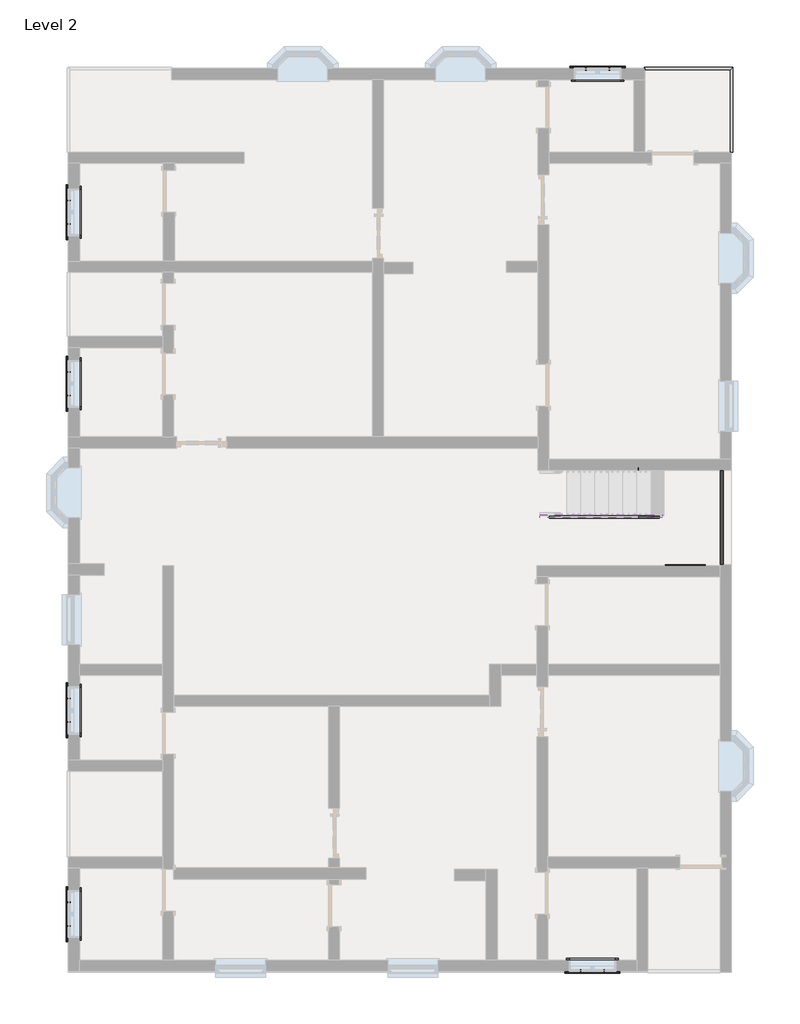
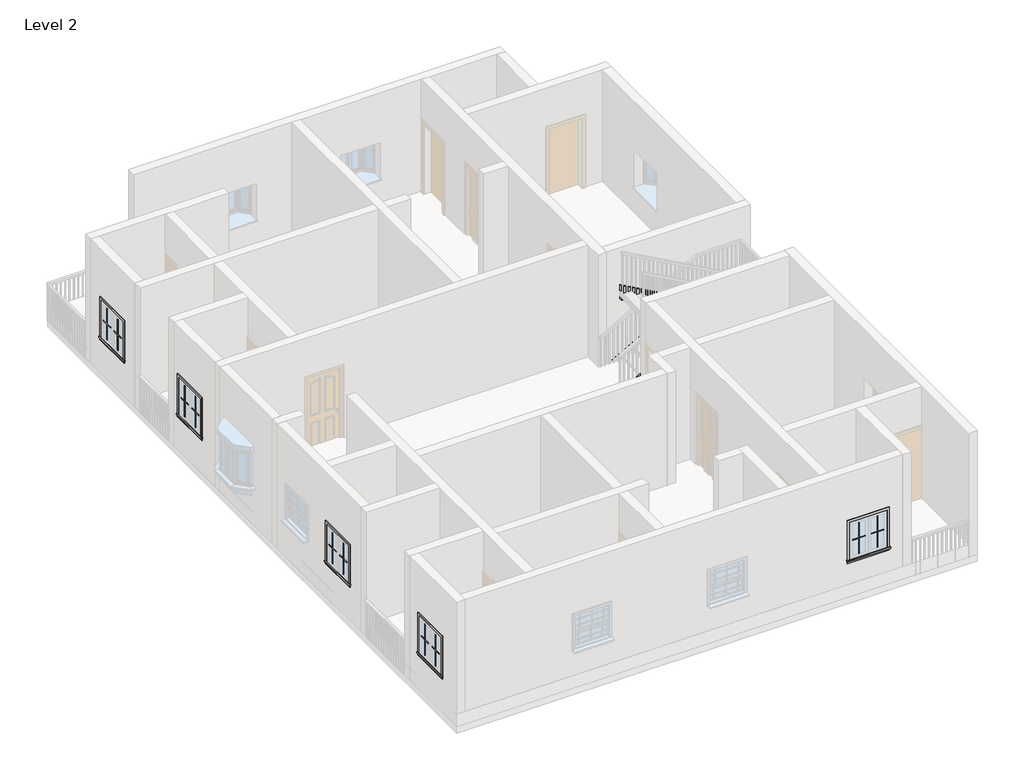
# One storey, part 4 of 4: 24 proxies, 5 members, 1 railing.
"""IFC4 building model written with IfcOpenShell, lengths in millimetres."""

from ifc_helpers import new_model, si_unit, frame, origin, place, context, project, spatial, polyline, outline, extrude, faceted_brep, transform, mapped, element, save
from components import muntin_pattern_2x2_muntin_pattern_2x2_b3fe6957, muntin_pattern_2x2_muntin_pattern_2x2_3e0ecaf2, trim_window_exterior_flat_with_sill_41619996, trim_window_interior_flat_picture_frame_51c85655

model = new_model("IFC4")

# Units and contexts
model_context = context("Model", 3, world=origin())
ifc_project = project(units=[si_unit("LENGTHUNIT", "METRE", prefix="MILLI")], contexts=[model_context])

# Site, building, storey
site = spatial("IfcSite", under=ifc_project)
building = spatial("IfcBuilding", under=site)
storey = spatial("IfcBuildingStorey", under=building, Name="Level 2", Elevation=3048.0)

# Proxies
placement = place(None, origin())
muntin_pattern_2x2_muntin_pattern_2x2_shape = muntin_pattern_2x2_muntin_pattern_2x2_b3fe6957(model_context)
element("IfcBuildingElementProxy", 1, Name="Muntin Pattern_2x2 : Muntin Pattern_2x2", ObjectType="Muntin Pattern_2x2 : Muntin Pattern_2x2", at=placement, inside=storey, context=model_context, shape_type="MappedRepresentation", body=[
    mapped(muntin_pattern_2x2_muntin_pattern_2x2_shape, transform((-7038.4808717, 5489.0318597, 4032.25), x_axis=(0.0, 1.0, 0.0), y_axis=(-1.0, 0.0, 0.0), z_axis=(0.0, 0.0, 1.0))),
])
element("IfcBuildingElementProxy", 2, Name="Muntin Pattern_2x2 : Muntin Pattern_2x2", ObjectType="Muntin Pattern_2x2 : Muntin Pattern_2x2", at=placement, inside=storey, context=model_context, shape_type="MappedRepresentation", body=[
    mapped(muntin_pattern_2x2_muntin_pattern_2x2_shape, transform((-7038.4808717, 2366.9422293, 4032.25), x_axis=(0.0, 1.0, 0.0), y_axis=(-1.0, 0.0, 0.0), z_axis=(0.0, 0.0, 1.0))),
])
element("IfcBuildingElementProxy", 3, Name="Muntin Pattern_2x2 : Muntin Pattern_2x2", ObjectType="Muntin Pattern_2x2 : Muntin Pattern_2x2", at=placement, inside=storey, context=model_context, shape_type="MappedRepresentation", body=[
    mapped(muntin_pattern_2x2_muntin_pattern_2x2_shape, transform((2376.9816283, 8312.1297293, 4032.25), x_axis=(1.0, 0.0, 0.0), y_axis=(0.0, 1.0, 0.0), z_axis=(0.0, 0.0, 1.0))),
])
element("IfcBuildingElementProxy", 4, Name="Muntin Pattern_2x2 : Muntin Pattern_2x2", ObjectType="Muntin Pattern_2x2 : Muntin Pattern_2x2", at=placement, inside=storey, context=model_context, shape_type="MappedRepresentation", body=[
    mapped(muntin_pattern_2x2_muntin_pattern_2x2_shape, transform((2710.3566283, -8102.6202707, 4032.25), x_axis=(-1.0, 0.0, 0.0), y_axis=(0.0, -1.0, 0.0), z_axis=(0.0, 0.0, 1.0))),
])
element("IfcBuildingElementProxy", 5, Name="Muntin Pattern_2x2 : Muntin Pattern_2x2", ObjectType="Muntin Pattern_2x2 : Muntin Pattern_2x2", at=placement, inside=storey, context=model_context, shape_type="MappedRepresentation", body=[
    mapped(muntin_pattern_2x2_muntin_pattern_2x2_shape, transform((-7038.4808717, -7285.0577707, 4032.25), x_axis=(0.0, 1.0, 0.0), y_axis=(-1.0, 0.0, 0.0), z_axis=(0.0, 0.0, 1.0))),
])
element("IfcBuildingElementProxy", 6, Name="Muntin Pattern_2x2 : Muntin Pattern_2x2", ObjectType="Muntin Pattern_2x2 : Muntin Pattern_2x2", at=placement, inside=storey, context=model_context, shape_type="MappedRepresentation", body=[
    mapped(muntin_pattern_2x2_muntin_pattern_2x2_shape, transform((-7038.4808717, -3576.6577707, 4032.25), x_axis=(0.0, 1.0, 0.0), y_axis=(-1.0, 0.0, 0.0), z_axis=(0.0, 0.0, 1.0))),
])
muntin_pattern_2x2_muntin_pattern_2x2_2_shape = muntin_pattern_2x2_muntin_pattern_2x2_3e0ecaf2(model_context)
element("IfcBuildingElementProxy", 7, Name="Muntin Pattern_2x2 : Muntin Pattern_2x2", ObjectType="Muntin Pattern_2x2 : Muntin Pattern_2x2", at=placement, inside=storey, context=model_context, shape_type="MappedRepresentation", body=[
    mapped(muntin_pattern_2x2_muntin_pattern_2x2_2_shape, transform((-7038.4808717, 5917.6568597, 4032.25), x_axis=(0.0, -1.0, 0.0), y_axis=(1.0, 0.0, 0.0), z_axis=(0.0, 0.0, 1.0))),
])
element("IfcBuildingElementProxy", 8, Name="Muntin Pattern_2x2 : Muntin Pattern_2x2", ObjectType="Muntin Pattern_2x2 : Muntin Pattern_2x2", at=placement, inside=storey, context=model_context, shape_type="MappedRepresentation", body=[
    mapped(muntin_pattern_2x2_muntin_pattern_2x2_2_shape, transform((-7038.4808717, 2795.5672293, 4032.25), x_axis=(0.0, -1.0, 0.0), y_axis=(1.0, 0.0, 0.0), z_axis=(0.0, 0.0, 1.0))),
])
element("IfcBuildingElementProxy", 9, Name="Muntin Pattern_2x2 : Muntin Pattern_2x2", ObjectType="Muntin Pattern_2x2 : Muntin Pattern_2x2", at=placement, inside=storey, context=model_context, shape_type="MappedRepresentation", body=[
    mapped(muntin_pattern_2x2_muntin_pattern_2x2_2_shape, transform((2805.6066283, 8312.1297293, 4032.25), x_axis=(-1.0, 0.0, 0.0), y_axis=(0.0, -1.0, 0.0), z_axis=(0.0, 0.0, 1.0))),
])
element("IfcBuildingElementProxy", 10, Name="Muntin Pattern_2x2 : Muntin Pattern_2x2", ObjectType="Muntin Pattern_2x2 : Muntin Pattern_2x2", at=placement, inside=storey, context=model_context, shape_type="MappedRepresentation", body=[
    mapped(muntin_pattern_2x2_muntin_pattern_2x2_2_shape, transform((2281.7316283, -8102.6202707, 4032.25), x_axis=(1.0, 0.0, 0.0), y_axis=(0.0, 1.0, 0.0), z_axis=(0.0, 0.0, 1.0))),
])
element("IfcBuildingElementProxy", 11, Name="Muntin Pattern_2x2 : Muntin Pattern_2x2", ObjectType="Muntin Pattern_2x2 : Muntin Pattern_2x2", at=placement, inside=storey, context=model_context, shape_type="MappedRepresentation", body=[
    mapped(muntin_pattern_2x2_muntin_pattern_2x2_2_shape, transform((-7038.4808717, -6856.4327707, 4032.25), x_axis=(0.0, -1.0, 0.0), y_axis=(1.0, 0.0, 0.0), z_axis=(0.0, 0.0, 1.0))),
])
element("IfcBuildingElementProxy", 12, Name="Muntin Pattern_2x2 : Muntin Pattern_2x2", ObjectType="Muntin Pattern_2x2 : Muntin Pattern_2x2", at=placement, inside=storey, context=model_context, shape_type="MappedRepresentation", body=[
    mapped(muntin_pattern_2x2_muntin_pattern_2x2_2_shape, transform((-7038.4808717, -3148.0327707, 4032.25), x_axis=(0.0, -1.0, 0.0), y_axis=(1.0, 0.0, 0.0), z_axis=(0.0, 0.0, 1.0))),
])
trim_window_exterior_flat_with_sill_shape = trim_window_exterior_flat_with_sill_41619996(model_context)
element("IfcBuildingElementProxy", 13, Name="Trim-Window-Exterior-Flat : with Sill", ObjectType="Trim-Window-Exterior-Flat : with Sill", at=placement, inside=storey, context=model_context, shape_type="MappedRepresentation", body=[
    mapped(trim_window_exterior_flat_with_sill_shape, transform((-7048.0058717, 5703.3443597, 4876.8), x_axis=(0.0, -1.0, 0.0), y_axis=(0.0, 0.0, 1.0), z_axis=(-1.0, 0.0, 0.0))),
])
element("IfcBuildingElementProxy", 14, Name="Trim-Window-Exterior-Flat : with Sill", ObjectType="Trim-Window-Exterior-Flat : with Sill", at=placement, inside=storey, context=model_context, shape_type="MappedRepresentation", body=[
    mapped(trim_window_exterior_flat_with_sill_shape, transform((-7048.0058717, 2581.2547293, 4876.8), x_axis=(0.0, -1.0, 0.0), y_axis=(0.0, 0.0, 1.0), z_axis=(-1.0, 0.0, 0.0))),
])
element("IfcBuildingElementProxy", 15, Name="Trim-Window-Exterior-Flat : with Sill", ObjectType="Trim-Window-Exterior-Flat : with Sill", at=placement, inside=storey, context=model_context, shape_type="MappedRepresentation", body=[
    mapped(trim_window_exterior_flat_with_sill_shape, transform((2591.2941283, 8321.6547293, 4876.8), x_axis=(-1.0, 0.0, 0.0), y_axis=(0.0, 0.0, 1.0), z_axis=(0.0, 1.0, 0.0))),
])
element("IfcBuildingElementProxy", 16, Name="Trim-Window-Exterior-Flat : with Sill", ObjectType="Trim-Window-Exterior-Flat : with Sill", at=placement, inside=storey, context=model_context, shape_type="MappedRepresentation", body=[
    mapped(trim_window_exterior_flat_with_sill_shape, transform((2496.0441283, -8112.1452707, 4876.8), x_axis=(1.0, 0.0, 0.0), y_axis=(0.0, 0.0, 1.0), z_axis=(0.0, -1.0, 0.0))),
])
element("IfcBuildingElementProxy", 17, Name="Trim-Window-Exterior-Flat : with Sill", ObjectType="Trim-Window-Exterior-Flat : with Sill", at=placement, inside=storey, context=model_context, shape_type="MappedRepresentation", body=[
    mapped(trim_window_exterior_flat_with_sill_shape, transform((-7048.0058717, -7070.7452707, 4876.8), x_axis=(0.0, -1.0, 0.0), y_axis=(0.0, 0.0, 1.0), z_axis=(-1.0, 0.0, 0.0))),
])
element("IfcBuildingElementProxy", 18, Name="Trim-Window-Exterior-Flat : with Sill", ObjectType="Trim-Window-Exterior-Flat : with Sill", at=placement, inside=storey, context=model_context, shape_type="MappedRepresentation", body=[
    mapped(trim_window_exterior_flat_with_sill_shape, transform((-7048.0058717, -3362.3452707, 4876.8), x_axis=(0.0, -1.0, 0.0), y_axis=(0.0, 0.0, 1.0), z_axis=(-1.0, 0.0, 0.0))),
])
trim_window_interior_flat_picture_frame_shape = trim_window_interior_flat_picture_frame_51c85655(model_context)
element("IfcBuildingElementProxy", 19, Name="Trim-Window-Interior-Flat : Picture Frame", ObjectType="Trim-Window-Interior-Flat : Picture Frame", at=placement, inside=storey, context=model_context, shape_type="MappedRepresentation", body=[
    mapped(trim_window_interior_flat_picture_frame_shape, transform((-6844.8058717, 5703.3443597, 4876.8), x_axis=(0.0, 1.0, 0.0), y_axis=(0.0, 0.0, 1.0), z_axis=(1.0, 0.0, 0.0))),
])
element("IfcBuildingElementProxy", 20, Name="Trim-Window-Interior-Flat : Picture Frame", ObjectType="Trim-Window-Interior-Flat : Picture Frame", at=placement, inside=storey, context=model_context, shape_type="MappedRepresentation", body=[
    mapped(trim_window_interior_flat_picture_frame_shape, transform((-6844.8058717, 2581.2547293, 4876.8), x_axis=(0.0, 1.0, 0.0), y_axis=(0.0, 0.0, 1.0), z_axis=(1.0, 0.0, 0.0))),
])
element("IfcBuildingElementProxy", 21, Name="Trim-Window-Interior-Flat : Picture Frame", ObjectType="Trim-Window-Interior-Flat : Picture Frame", at=placement, inside=storey, context=model_context, shape_type="MappedRepresentation", body=[
    mapped(trim_window_interior_flat_picture_frame_shape, transform((2591.2941283, 8118.4547293, 4876.8), x_axis=(1.0, 0.0, 0.0), y_axis=(0.0, 0.0, 1.0), z_axis=(0.0, -1.0, 0.0))),
])
element("IfcBuildingElementProxy", 22, Name="Trim-Window-Interior-Flat : Picture Frame", ObjectType="Trim-Window-Interior-Flat : Picture Frame", at=placement, inside=storey, context=model_context, shape_type="MappedRepresentation", body=[
    mapped(trim_window_interior_flat_picture_frame_shape, transform((2496.0441283, -7908.9452707, 4876.8), x_axis=(-1.0, 0.0, 0.0), y_axis=(0.0, 0.0, 1.0), z_axis=(0.0, 1.0, 0.0))),
])
element("IfcBuildingElementProxy", 23, Name="Trim-Window-Interior-Flat : Picture Frame", ObjectType="Trim-Window-Interior-Flat : Picture Frame", at=placement, inside=storey, context=model_context, shape_type="MappedRepresentation", body=[
    mapped(trim_window_interior_flat_picture_frame_shape, transform((-6844.8058717, -7070.7452707, 4876.8), x_axis=(0.0, 1.0, 0.0), y_axis=(0.0, 0.0, 1.0), z_axis=(1.0, 0.0, 0.0))),
])
element("IfcBuildingElementProxy", 24, Name="Trim-Window-Interior-Flat : Picture Frame", ObjectType="Trim-Window-Interior-Flat : Picture Frame", at=placement, inside=storey, context=model_context, shape_type="MappedRepresentation", body=[
    mapped(trim_window_interior_flat_picture_frame_shape, transform((-6844.8058717, -3362.3452707, 4876.8), x_axis=(0.0, 1.0, 0.0), y_axis=(0.0, 0.0, 1.0), z_axis=(1.0, 0.0, 0.0))),
])

# Members
element("IfcMember", 25, ObjectType="Stringer - 2\" Width", at=placement, inside=storey, context=model_context, shape_type="SweptSolid", body=[
    extrude(outline(polyline([(3258.6757607, 1537.1941283), (3048.0, 1537.1941283), (3048.0, 1786.1766781), (4495.8, 4407.1563102), (4495.8, 3776.7834593), (3258.6757607, 1537.1941283)])), frame((0.0, 1006.4547293, 0.0), z_axis=(0.0, 1.0, 0.0), x_axis=(0.0, 0.0, 1.0)), (0.0, 0.0, 1.0), 50.8),
])
element("IfcMember", 26, ObjectType="Stringer - 2\" Width", at=placement, inside=storey, context=model_context, shape_type="SweptSolid", body=[
    extrude(outline(polyline([(4826.4941283, 1057.2547293), (4877.2941283, 1057.2547293), (4877.2941283, -714.2964201), (4826.4941283, -714.2964201), (4826.4941283, 1057.2547293)])), frame((0.0, 0.0, 4191.0), z_axis=(0.0, 0.0, 1.0), x_axis=(1.0, 0.0, 0.0)), (0.0, 0.0, 1.0), 304.8),
])
element("IfcMember", 27, ObjectType="Stringer - 2\" Width", at=placement, inside=storey, context=model_context, shape_type="SweptSolid", body=[
    extrude(outline(polyline([(4191.0, 4555.0346706), (5858.0215532, 1537.1941283), (5509.8106009, 1537.1941283), (4191.0, 3924.6618197), (4191.0, 4555.0346706)])), frame((0.0, -765.0964201, 0.0), z_axis=(0.0, 1.0, 0.0), x_axis=(0.0, 0.0, 1.0)), (0.0, 0.0, 1.0), 50.8),
])
element("IfcMember", 28, ObjectType="Stringer - 2\" Width", at=placement, inside=storey, context=model_context, shape_type="SweptSolid", body=[
    extrude(outline(polyline([(3258.6757607, 1537.1941283), (3048.0, 1537.1941283), (3048.0, 1786.1766781), (4113.4963497, 3715.0648053), (4461.7073019, 3715.0648053), (3258.6757607, 1537.1941283)])), frame((0.0, 130.1547293, 0.0), z_axis=(0.0, 1.0, 0.0), x_axis=(0.0, 0.0, 1.0)), (0.0, 0.0, 1.0), 50.8),
])
element("IfcMember", 29, ObjectType="Stringer - 2\" Width", at=placement, inside=storey, context=model_context, shape_type="SweptSolid", body=[
    extrude(outline(polyline([(4278.7177047, 3765.8648053), (4626.928657, 3765.8648053), (5858.0215532, 1537.1941283), (5509.8106009, 1537.1941283), (4278.7177047, 3765.8648053)])), frame((0.0, 142.8547293, 0.0), z_axis=(0.0, 1.0, 0.0), x_axis=(0.0, 0.0, 1.0)), (0.0, 0.0, 1.0), 50.8),
])

# Railing
element("IfcRailing", 30, ObjectType="Handrail - Rectangular", at=placement, inside=storey, context=model_context, shape_type="SolidModel", body=[
    faceted_brep([(3442.1941283, 8347.0547293, 3962.4), (3442.1941283, 8347.0547293, 3911.6), (3442.1941283, 8296.2547293, 3911.6), (3442.1941283, 8296.2547293, 3962.4), (5055.0941283, 8347.0547293, 3962.4), (5055.0941283, 8347.0547293, 3911.6), (5004.2941283, 8296.2547293, 3911.6), (5004.2941283, 8296.2547293, 3962.4), (5055.0941283, 6797.6547293, 3962.4), (5004.2941283, 6797.6547293, 3962.4), (5004.2941283, 6797.6547293, 3911.6), (5055.0941283, 6797.6547293, 3911.6)], [[[0, 1, 2, 3]], [[1, 0, 4, 5]], [[2, 1, 5, 6]], [[3, 2, 6, 7]], [[0, 3, 7, 4]], [[8, 9, 10, 11]], [[5, 4, 8, 11]], [[6, 5, 11, 10]], [[7, 6, 10, 9]], [[4, 7, 9, 8]]]),
    extrude(outline(polyline([(5020.1691283, 6908.7797293), (5039.2191283, 6908.7797293), (5039.2191283, 6889.7297293), (5020.1691283, 6889.7297293), (5020.1691283, 6908.7797293)])), frame((0.0, 0.0, 3048.0), z_axis=(0.0, 0.0, 1.0), x_axis=(1.0, 0.0, 0.0)), (0.0, 0.0, 1.0), 863.6),
    extrude(outline(polyline([(5020.1691283, 7010.3797293), (5039.2191283, 7010.3797293), (5039.2191283, 6991.3297293), (5020.1691283, 6991.3297293), (5020.1691283, 7010.3797293)])), frame((0.0, 0.0, 3048.0), z_axis=(0.0, 0.0, 1.0), x_axis=(1.0, 0.0, 0.0)), (0.0, 0.0, 1.0), 863.6),
    extrude(outline(polyline([(5020.1691283, 7111.9797293), (5039.2191283, 7111.9797293), (5039.2191283, 7092.9297293), (5020.1691283, 7092.9297293), (5020.1691283, 7111.9797293)])), frame((0.0, 0.0, 3048.0), z_axis=(0.0, 0.0, 1.0), x_axis=(1.0, 0.0, 0.0)), (0.0, 0.0, 1.0), 863.6),
    extrude(outline(polyline([(5020.1691283, 7213.5797293), (5039.2191283, 7213.5797293), (5039.2191283, 7194.5297293), (5020.1691283, 7194.5297293), (5020.1691283, 7213.5797293)])), frame((0.0, 0.0, 3048.0), z_axis=(0.0, 0.0, 1.0), x_axis=(1.0, 0.0, 0.0)), (0.0, 0.0, 1.0), 863.6),
    extrude(outline(polyline([(5020.1691283, 7315.1797293), (5039.2191283, 7315.1797293), (5039.2191283, 7296.1297293), (5020.1691283, 7296.1297293), (5020.1691283, 7315.1797293)])), frame((0.0, 0.0, 3048.0), z_axis=(0.0, 0.0, 1.0), x_axis=(1.0, 0.0, 0.0)), (0.0, 0.0, 1.0), 863.6),
    extrude(outline(polyline([(5020.1691283, 7416.7797293), (5039.2191283, 7416.7797293), (5039.2191283, 7397.7297293), (5020.1691283, 7397.7297293), (5020.1691283, 7416.7797293)])), frame((0.0, 0.0, 3048.0), z_axis=(0.0, 0.0, 1.0), x_axis=(1.0, 0.0, 0.0)), (0.0, 0.0, 1.0), 863.6),
    extrude(outline(polyline([(5020.1691283, 7518.3797293), (5039.2191283, 7518.3797293), (5039.2191283, 7499.3297293), (5020.1691283, 7499.3297293), (5020.1691283, 7518.3797293)])), frame((0.0, 0.0, 3048.0), z_axis=(0.0, 0.0, 1.0), x_axis=(1.0, 0.0, 0.0)), (0.0, 0.0, 1.0), 863.6),
    extrude(outline(polyline([(5020.1691283, 7619.9797293), (5039.2191283, 7619.9797293), (5039.2191283, 7600.9297293), (5020.1691283, 7600.9297293), (5020.1691283, 7619.9797293)])), frame((0.0, 0.0, 3048.0), z_axis=(0.0, 0.0, 1.0), x_axis=(1.0, 0.0, 0.0)), (0.0, 0.0, 1.0), 863.6),
    extrude(outline(polyline([(5020.1691283, 7721.5797293), (5039.2191283, 7721.5797293), (5039.2191283, 7702.5297293), (5020.1691283, 7702.5297293), (5020.1691283, 7721.5797293)])), frame((0.0, 0.0, 3048.0), z_axis=(0.0, 0.0, 1.0), x_axis=(1.0, 0.0, 0.0)), (0.0, 0.0, 1.0), 863.6),
    extrude(outline(polyline([(5020.1691283, 7823.1797293), (5039.2191283, 7823.1797293), (5039.2191283, 7804.1297293), (5020.1691283, 7804.1297293), (5020.1691283, 7823.1797293)])), frame((0.0, 0.0, 3048.0), z_axis=(0.0, 0.0, 1.0), x_axis=(1.0, 0.0, 0.0)), (0.0, 0.0, 1.0), 863.6),
    extrude(outline(polyline([(5020.1691283, 7924.7797293), (5039.2191283, 7924.7797293), (5039.2191283, 7905.7297293), (5020.1691283, 7905.7297293), (5020.1691283, 7924.7797293)])), frame((0.0, 0.0, 3048.0), z_axis=(0.0, 0.0, 1.0), x_axis=(1.0, 0.0, 0.0)), (0.0, 0.0, 1.0), 863.6),
    extrude(outline(polyline([(5020.1691283, 8026.3797293), (5039.2191283, 8026.3797293), (5039.2191283, 8007.3297293), (5020.1691283, 8007.3297293), (5020.1691283, 8026.3797293)])), frame((0.0, 0.0, 3048.0), z_axis=(0.0, 0.0, 1.0), x_axis=(1.0, 0.0, 0.0)), (0.0, 0.0, 1.0), 863.6),
    extrude(outline(polyline([(5020.1691283, 8127.9797293), (5039.2191283, 8127.9797293), (5039.2191283, 8108.9297293), (5020.1691283, 8108.9297293), (5020.1691283, 8127.9797293)])), frame((0.0, 0.0, 3048.0), z_axis=(0.0, 0.0, 1.0), x_axis=(1.0, 0.0, 0.0)), (0.0, 0.0, 1.0), 863.6),
    extrude(outline(polyline([(5020.1691283, 8229.5797293), (5039.2191283, 8229.5797293), (5039.2191283, 8210.5297293), (5020.1691283, 8210.5297293), (5020.1691283, 8229.5797293)])), frame((0.0, 0.0, 3048.0), z_axis=(0.0, 0.0, 1.0), x_axis=(1.0, 0.0, 0.0)), (0.0, 0.0, 1.0), 863.6),
    extrude(outline(polyline([(4956.6691283, 8312.1297293), (4956.6691283, 8331.1797293), (4975.7191283, 8331.1797293), (4975.7191283, 8312.1297293), (4956.6691283, 8312.1297293)])), frame((0.0, 0.0, 3048.0), z_axis=(0.0, 0.0, 1.0), x_axis=(1.0, 0.0, 0.0)), (0.0, 0.0, 1.0), 863.6),
    extrude(outline(polyline([(4855.0691283, 8312.1297293), (4855.0691283, 8331.1797293), (4874.1191283, 8331.1797293), (4874.1191283, 8312.1297293), (4855.0691283, 8312.1297293)])), frame((0.0, 0.0, 3048.0), z_axis=(0.0, 0.0, 1.0), x_axis=(1.0, 0.0, 0.0)), (0.0, 0.0, 1.0), 863.6),
    extrude(outline(polyline([(4753.4691283, 8312.1297293), (4753.4691283, 8331.1797293), (4772.5191283, 8331.1797293), (4772.5191283, 8312.1297293), (4753.4691283, 8312.1297293)])), frame((0.0, 0.0, 3048.0), z_axis=(0.0, 0.0, 1.0), x_axis=(1.0, 0.0, 0.0)), (0.0, 0.0, 1.0), 863.6),
    extrude(outline(polyline([(4651.8691283, 8312.1297293), (4651.8691283, 8331.1797293), (4670.9191283, 8331.1797293), (4670.9191283, 8312.1297293), (4651.8691283, 8312.1297293)])), frame((0.0, 0.0, 3048.0), z_axis=(0.0, 0.0, 1.0), x_axis=(1.0, 0.0, 0.0)), (0.0, 0.0, 1.0), 863.6),
    extrude(outline(polyline([(4550.2691283, 8312.1297293), (4550.2691283, 8331.1797293), (4569.3191283, 8331.1797293), (4569.3191283, 8312.1297293), (4550.2691283, 8312.1297293)])), frame((0.0, 0.0, 3048.0), z_axis=(0.0, 0.0, 1.0), x_axis=(1.0, 0.0, 0.0)), (0.0, 0.0, 1.0), 863.6),
    extrude(outline(polyline([(4448.6691283, 8312.1297293), (4448.6691283, 8331.1797293), (4467.7191283, 8331.1797293), (4467.7191283, 8312.1297293), (4448.6691283, 8312.1297293)])), frame((0.0, 0.0, 3048.0), z_axis=(0.0, 0.0, 1.0), x_axis=(1.0, 0.0, 0.0)), (0.0, 0.0, 1.0), 863.6),
    extrude(outline(polyline([(4347.0691283, 8312.1297293), (4347.0691283, 8331.1797293), (4366.1191283, 8331.1797293), (4366.1191283, 8312.1297293), (4347.0691283, 8312.1297293)])), frame((0.0, 0.0, 3048.0), z_axis=(0.0, 0.0, 1.0), x_axis=(1.0, 0.0, 0.0)), (0.0, 0.0, 1.0), 863.6),
    extrude(outline(polyline([(4245.4691283, 8312.1297293), (4245.4691283, 8331.1797293), (4264.5191283, 8331.1797293), (4264.5191283, 8312.1297293), (4245.4691283, 8312.1297293)])), frame((0.0, 0.0, 3048.0), z_axis=(0.0, 0.0, 1.0), x_axis=(1.0, 0.0, 0.0)), (0.0, 0.0, 1.0), 863.6),
    extrude(outline(polyline([(4143.8691283, 8312.1297293), (4143.8691283, 8331.1797293), (4162.9191283, 8331.1797293), (4162.9191283, 8312.1297293), (4143.8691283, 8312.1297293)])), frame((0.0, 0.0, 3048.0), z_axis=(0.0, 0.0, 1.0), x_axis=(1.0, 0.0, 0.0)), (0.0, 0.0, 1.0), 863.6),
    extrude(outline(polyline([(4042.2691283, 8312.1297293), (4042.2691283, 8331.1797293), (4061.3191283, 8331.1797293), (4061.3191283, 8312.1297293), (4042.2691283, 8312.1297293)])), frame((0.0, 0.0, 3048.0), z_axis=(0.0, 0.0, 1.0), x_axis=(1.0, 0.0, 0.0)), (0.0, 0.0, 1.0), 863.6),
    extrude(outline(polyline([(3940.6691283, 8312.1297293), (3940.6691283, 8331.1797293), (3959.7191283, 8331.1797293), (3959.7191283, 8312.1297293), (3940.6691283, 8312.1297293)])), frame((0.0, 0.0, 3048.0), z_axis=(0.0, 0.0, 1.0), x_axis=(1.0, 0.0, 0.0)), (0.0, 0.0, 1.0), 863.6),
    extrude(outline(polyline([(3839.0691283, 8312.1297293), (3839.0691283, 8331.1797293), (3858.1191283, 8331.1797293), (3858.1191283, 8312.1297293), (3839.0691283, 8312.1297293)])), frame((0.0, 0.0, 3048.0), z_axis=(0.0, 0.0, 1.0), x_axis=(1.0, 0.0, 0.0)), (0.0, 0.0, 1.0), 863.6),
    extrude(outline(polyline([(3737.4691283, 8312.1297293), (3737.4691283, 8331.1797293), (3756.5191283, 8331.1797293), (3756.5191283, 8312.1297293), (3737.4691283, 8312.1297293)])), frame((0.0, 0.0, 3048.0), z_axis=(0.0, 0.0, 1.0), x_axis=(1.0, 0.0, 0.0)), (0.0, 0.0, 1.0), 863.6),
    extrude(outline(polyline([(3635.8691283, 8312.1297293), (3635.8691283, 8331.1797293), (3654.9191283, 8331.1797293), (3654.9191283, 8312.1297293), (3635.8691283, 8312.1297293)])), frame((0.0, 0.0, 3048.0), z_axis=(0.0, 0.0, 1.0), x_axis=(1.0, 0.0, 0.0)), (0.0, 0.0, 1.0), 863.6),
    extrude(outline(polyline([(3534.2691283, 8312.1297293), (3534.2691283, 8331.1797293), (3553.3191283, 8331.1797293), (3553.3191283, 8312.1297293), (3534.2691283, 8312.1297293)])), frame((0.0, 0.0, 3048.0), z_axis=(0.0, 0.0, 1.0), x_axis=(1.0, 0.0, 0.0)), (0.0, 0.0, 1.0), 863.6),
    extrude(outline(polyline([(5020.1691283, 8312.1297293), (5020.1691283, 8331.1797293), (5039.2191283, 8331.1797293), (5039.2191283, 8312.1297293), (5020.1691283, 8312.1297293)])), frame((0.0, 0.0, 3048.0), z_axis=(0.0, 0.0, 1.0), x_axis=(1.0, 0.0, 0.0)), (0.0, 0.0, 1.0), 863.6),
    extrude(outline(polyline([(5020.1691283, 6816.7047293), (5039.2191283, 6816.7047293), (5039.2191283, 6797.6547293), (5020.1691283, 6797.6547293), (5020.1691283, 6816.7047293)])), frame((0.0, 0.0, 3048.0), z_axis=(0.0, 0.0, 1.0), x_axis=(1.0, 0.0, 0.0)), (0.0, 0.0, 1.0), 863.6),
    extrude(outline(polyline([(3442.1941283, 8312.1297293), (3442.1941283, 8331.1797293), (3461.2441283, 8331.1797293), (3461.2441283, 8312.1297293), (3442.1941283, 8312.1297293)])), frame((0.0, 0.0, 3048.0), z_axis=(0.0, 0.0, 1.0), x_axis=(1.0, 0.0, 0.0)), (0.0, 0.0, 1.0), 863.6),
])

save(model, "model.ifc")

# Revit data of these elements
# Type "Muntin Pattern_2x2 : Muntin Pattern_2x2"
#   Width [instance default] = 4' - 0"
#   Thickness = 0' - 0 1/2"
#   Height [instance default] = 4' - 0"
#   Distance = 0' - 0 3/4"
#   Interior Material [instance default] = none
#   Exterior Material [instance default] = none
#   Default Elevation = 0
# Type "Trim-Window-Exterior-Flat : with Sill"
#   Trim Width = 0' - 2 1/4"
#   Trim Thickness_Picture Frame = 0' - 1 1/4"
#   Trim Thickness_with Sill = 0' - 0 3/4"
#   Sill Thickness = 0' - 1 1/4"
#   Opening Width [instance default] = 2' - 0"
#   Opening Height [instance default] = 3' - 0"
#   Default Elevation = 4' - 0"
#   Sill = yes
#   Picture Frame = no
#   Trim Material [instance default] = none
# Type "Trim-Window-Interior-Flat : Picture Frame"
#   Trim Thickness_Picture Frame = 0' - 1 1/4"
#   Trim Width = 0' - 2 1/4"
#   Trim Thickness_with Sill = 0' - 0 3/4"
#   Sill Thickness = 0' - 1 1/4"
#   Opening Width [instance default] = 2' - 0"
#   Opening Height [instance default] = 3' - 0"
#   Default Elevation = 4' - 0"
#   Sill = no
#   Picture Frame = yes
#   Trim Material [instance default] = none
# Type "Handrail - Rectangular"
#   Assembly Code = "C2010400"
#   built-in parameter 1008612 = 0.0416667 (stored number, unit not read)
#   built-in parameter 1008611 = 0.0416667 (stored number, unit not read)
#   built-in parameter 1008609 = 0.333333 (stored number, unit not read)
#   built-in parameter 1008604 = 0.166667 (stored number, unit not read)
#   built-in parameter 1008603 = 0.166667 (stored number, unit not read)
#   Railing Height = 3' - 0"
#   built-in parameter 1008630 = 2
#   built-in parameter 1008610 = 2
#   built-in parameter 1008618 = Baluster - Square : 3/4"
# Elements 1, 2, 3, 4, 5, 6, 7, 8, 9, 10, 11, 12 (IfcBuildingElementProxy, "Muntin Pattern_2x2 : Muntin Pattern_2x2")
#   Width = 0' - 11 5/8"
#   Height = 2' - 6 1/2"
#   Interior Material = Wood - Stained
#   Exterior Material = Clad - White
#   Phase Created = New Construction
#   Materials on its faces: "Clad - White", "Wood - Stained"
# Elements 13, 14, 15, 16, 17, 18 (IfcBuildingElementProxy, "Trim-Window-Exterior-Flat : with Sill")
#   Opening Width = 2' - 10"
#   Opening Height = 3' - 0"
#   Trim Material = Clad - White
#   Phase Created = New Construction
#   Materials on its faces: "Clad - White"
# Elements 19, 20, 21, 22, 23, 24 (IfcBuildingElementProxy, "Trim-Window-Interior-Flat : Picture Frame")
#   Opening Width = 2' - 10"
#   Opening Height = 3' - 0"
#   Trim Material = Wood - Stained
#   Phase Created = New Construction
#   Materials on its faces: "Wood - Stained"
# Elements 25, 27, 28, 29 (IfcMember, "Stringer - 2\" Width")
#   Phase Created = New Construction
# Element 26 (IfcMember, "Stringer - 2\" Width")
#   Phase Created = New Construction
#   Materials on its faces: "Render Material 41-165-0"
# Element 30 (IfcRailing, "Handrail - Rectangular")
#   Phase Created = New Construction
# Materials
#   "Clad - White": class "Wood", colour RGB 242 242 238, transparency 0, Cost = 0
#   "Wood - Stained": class "Wood", colour RGB 224 178 126, transparency 0, Cost = 0
#   "Render Material 41-165-0": colour RGB 41 165 0, transparency 0
